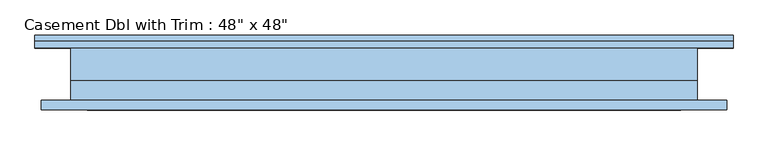
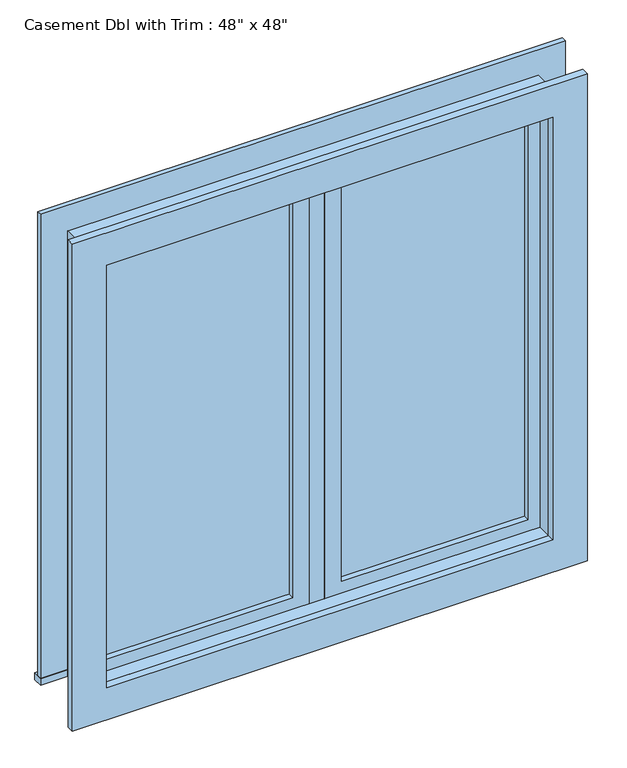
"""IFC4 building model written with IfcOpenShell, lengths in millimetres: window geometry."""

from ifc_helpers import new_model, si_unit, frame, origin, place, context, project, spatial, polyline, outline, extrude, source, transform, mapped, element, save


def window_90ef9153(model_context):
    return source(origin(), model_context, "Body", "SweptSolid", [
        extrude(outline(polyline([(63.5, 34.925), (546.1, 34.925), (546.1, 22.225), (63.5, 22.225), (63.5, 34.925)])), frame((0.0, 0.0, 977.9), z_axis=(0.0, 0.0, 1.0), x_axis=(1.0, 0.0, 0.0)), (0.0, 0.0, 1.0), 1092.2),
        extrude(outline(polyline([(2114.55, 19.05), (933.45, 19.05), (933.45, 590.55), (2114.55, 590.55), (2114.55, 19.05)]), holes=[polyline([(2070.1, 63.5), (2070.1, 546.1), (977.9, 546.1), (977.9, 63.5), (2070.1, 63.5)])]), frame((0.0, 6.35, 0.0), z_axis=(0.0, 1.0, 0.0), x_axis=(0.0, 0.0, 1.0)), (0.0, 0.0, 1.0), 44.45),
        extrude(outline(polyline([(19.05, 6.35), (-19.05, 6.35), (-19.05, 69.85), (19.05, 69.85), (19.05, 6.35)])), frame((0.0, 0.0, 933.45), z_axis=(0.0, 0.0, 1.0), x_axis=(1.0, 0.0, 0.0)), (0.0, 0.0, 1.0), 1181.1),
        extrude(outline(polyline([(-679.45, 95.25), (679.45, 95.25), (679.45, 69.85), (-679.45, 69.85), (-679.45, 95.25)])), frame((0.0, 0.0, 914.4), z_axis=(0.0, 0.0, 1.0), x_axis=(1.0, 0.0, 0.0)), (0.0, 0.0, 1.0), 19.05),
        extrude(outline(polyline([(2114.55, -590.55), (2114.55, 590.55), (933.45, 590.55), (933.45, 679.45), (2203.45, 679.45), (2203.45, -679.45), (933.45, -679.45), (933.45, -590.55), (2114.55, -590.55)])), frame((0.0, 69.85, 0.0), z_axis=(0.0, 1.0, 0.0), x_axis=(0.0, 0.0, 1.0)), (0.0, 0.0, 1.0), 12.7),
        extrude(outline(polyline([(2190.75, 666.75), (2190.75, -666.75), (857.25, -666.75), (857.25, 666.75), (2190.75, 666.75)]), holes=[polyline([(2101.85, 577.85), (946.15, 577.85), (946.15, -577.85), (2101.85, -577.85), (2101.85, 577.85)])]), frame((0.0, -50.8, 0.0), z_axis=(0.0, 1.0, 0.0), x_axis=(0.0, 0.0, 1.0)), (0.0, 0.0, 1.0), 19.05),
        extrude(outline(polyline([(-63.5, 22.225), (-546.1, 22.225), (-546.1, 34.925), (-63.5, 34.925), (-63.5, 22.225)])), frame((0.0, 0.0, 977.9), z_axis=(0.0, 0.0, 1.0), x_axis=(1.0, 0.0, 0.0)), (0.0, 0.0, 1.0), 1092.2),
        extrude(outline(polyline([(2114.55, -590.55), (933.45, -590.55), (933.45, -19.05), (2114.55, -19.05), (2114.55, -590.55)]), holes=[polyline([(2070.1, -546.1), (2070.1, -63.5), (977.9, -63.5), (977.9, -546.1), (2070.1, -546.1)])]), frame((0.0, 6.35, 0.0), z_axis=(0.0, 1.0, 0.0), x_axis=(0.0, 0.0, 1.0)), (0.0, 0.0, 1.0), 44.45),
        extrude(outline(polyline([(2133.6, -609.6), (914.4, -609.6), (914.4, 609.6), (2133.6, 609.6), (2133.6, -609.6)]), holes=[polyline([(2101.85, -577.85), (2101.85, 577.85), (946.15, 577.85), (946.15, -577.85), (2101.85, -577.85)])]), frame((0.0, -31.75, 0.0), z_axis=(0.0, 1.0, 0.0), x_axis=(0.0, 0.0, 1.0)), (0.0, 0.0, 1.0), 38.1),
        extrude(outline(polyline([(2133.6, 609.6), (2133.6, -609.6), (914.4, -609.6), (914.4, 609.6), (2133.6, 609.6)]), holes=[polyline([(2114.55, 590.55), (933.45, 590.55), (933.45, -590.55), (2114.55, -590.55), (2114.55, 590.55)])]), frame((0.0, 6.35, 0.0), z_axis=(0.0, 1.0, 0.0), x_axis=(0.0, 0.0, 1.0)), (0.0, 0.0, 1.0), 63.5),
    ])


if __name__ == "__main__":
    model = new_model("IFC4")
    model_context = context("Model", 3, world=origin())
    ifc_project = project(units=[si_unit("LENGTHUNIT", "METRE", prefix="MILLI")], contexts=[model_context])
    site = spatial("IfcSite", under=ifc_project)
    building = spatial("IfcBuilding", under=site)
    placement = place(None, origin())
    window_shape = window_90ef9153(model_context)
    element("IfcWindow", 1, ObjectType="Casement Dbl with Trim : 48\" x 48\"", at=placement, inside=building, context=model_context, shape_type="MappedRepresentation", body=[
        mapped(window_shape, transform((0.0, 0.0, 0.0), x_axis=(1.0, 0.0, 0.0), y_axis=(0.0, 1.0, 0.0), z_axis=(0.0, 0.0, 1.0))),
    ])
    save(model, "model.ifc")

# Revit data of these elements
# Type "Casement Dbl with Trim : 48\" x 48\""
#   Type Mark = "13"
#   Construction Type Id = "GSP4R"
#   Assembly Code = "B2020100"
#   Analytic Construction = "1/8 in Pilkington single glazing"
#   Visual Light Transmittance = 0.9
#   Solar Heat Gain Coefficient = 0.78
#   Heat Transfer Coefficient (U) = 0.6496 BTU/(h·ft²·°F)
#   Height = 4' - 0"
#   Default Sill Height = 3' - 0"
#   Trim Projection - Ext. = 0' - 0 1/2"
#   Trim Projection - Int. = 0' - 0 3/4"
#   Trim Width - Exterior = 0' - 3 1/2"
#   Trim Width - Interior = 0' - 3 1/2"
#   Width = 4' - 0"
#   Window Inset = 0' - 0 3/4"
#   Define Thermal Properties by = 1
#   Glass Pane Material = Glass
#   Sash Material = Sash
#   Trim Exterior Material = Trim
#   Trim Interior Material = Trim
#   Wall Closure = (empty or 0)
# Element 1 (IfcWindow, "Casement Dbl with Trim : 48\" x 48\"")
#   Materials on its faces: "Sash", "Trim", "Glass"
# Materials
#   "Glass": class "Glass", colour RGB 0 128 192, transparency 0.75, Description = "Soda Lime Glass", Cost = 0
#   "Sash": class "Wood", colour RGB 224 178 126, transparency 0
#   "Trim": class "Wood", colour RGB 224 178 126, transparency 0
